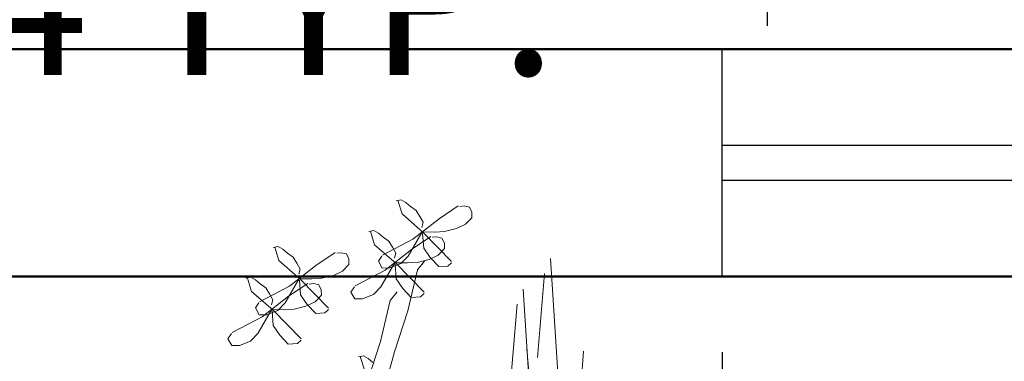
# Model space of a CAD drawing. Units: inches. Extents: x 89 to 490, y -59 to 378.
# Tile 6 of 20: x 300 to 339, y 1 to 15. Entities that reach past the tile are written whole.
import ezdxf

# ---------------------------------------------------------------- set-up
doc = ezdxf.new("R2010")
doc.units = ezdxf.units.IN
doc.header["$MEASUREMENT"] = 0
for name, color, linetype, lineweight in [('A-ANNO-DIMS', 2, 'Continuous', 18), ('L-PLNT', 94, 'Continuous', 18), ('Outer Walls', 12, 'Continuous', 50), ('Windows', 171, 'Continuous', 25)]:
    doc.layers.add(name, color=color, linetype=linetype, lineweight=lineweight)
doc.layers.add('fl', color=73, linetype='Continuous', lineweight=9, true_color=0xa3d166)
doc.styles.get("Standard").update_dxf_attribs({"font": 'arial.ttf'})
doc.dimstyles.get("Standard").update_dxf_attribs({"dimtxt": 6, "dimasz": 4, "dimexe": 3, "dimexo": 3, "dimgap": 0.09, "dimtad": 0, "dimtih": 1, "dimtoh": 1, "dimdec": 1, "dimzin": 0, "dimdsep": 46, "dimlunit": 3, "dimtxsty": 'Standard', "dimcen": 0.09, "dimadec": 0, "dimazin": 0, "dimtfac": 1, "dimtdec": 1, "dimtofl": 0, "dimtmove": 0, "dimatfit": 3, "dimfxl": 1, "dimtolj": 1, "dimtzin": 0, "dimarcsym": 0})

# ---------------------------------------------------------------- blocks, each defined once
blk = doc.blocks.new('Window')
for p, q in [((516.369, 95.253), (588.369, 95.253)), ((588.369, 93.853), (516.369, 93.853))]:
    blk.add_line(p, q)
blk.add_lwpolyline([(588.369, 99.053), (588.369, 90.053), (516.369, 90.053), (516.369, 99.053)], close=True)
blk = doc.blocks.new('Plantation')
at = {"layer": 'fl'}
for p, q in [((538.643, 42.607), (538.842, 42.647)), ((538.71, 42.613), (538.874, 42.084)), ((538.842, 42.647), (539.026, 42.541)), ((539.026, 42.541), (539.211, 42.38)), ((538.874, 42.084), (539.726, 41.335)), ((539.211, 42.38), (539.432, 42.22)), ((539.432, 42.22), (539.581, 41.986)), ((540.339, 41.891), (541.099, 42.403)), ((541.339, 42.399), (541.157, 42.378)), ((541.54, 42.348), (541.339, 42.399)), ((541.634, 42.149), (541.54, 42.348)), ((541.638, 41.931), (541.634, 42.149)), ((539.297, 41.078), (540.339, 41.891)), ((539.581, 41.986), (539.713, 41.752)), ((539.713, 41.752), (539.662, 41.55)), ((541.388, 41.672), (541.638, 41.931)), ((537.559, 41.389), (537.758, 41.429)), ((537.626, 41.395), (537.79, 40.866)), ((537.758, 41.429), (537.942, 41.323)), ((537.942, 41.323), (538.127, 41.162)), ((539.118, 40.412), (539.665, 41.35)), ((539.684, 41.314), (539.731, 40.732)), ((539.72, 41.369), (540.175, 41.359)), ((539.726, 41.335), (540.834, 40.206)), ((540.175, 41.359), (540.556, 41.384)), ((540.556, 41.384), (541.027, 41.501)), ((541.027, 41.501), (541.388, 41.672)), ((538.103, 40.454), (539.297, 41.078)), ((538.127, 41.162), (538.348, 41.002)), ((538.348, 41.002), (538.498, 40.768)), ((539.255, 40.673), (540.015, 41.185)), ((540.255, 41.181), (540.073, 41.16)), ((540.456, 41.13), (540.255, 41.181)), ((540.55, 40.931), (540.456, 41.13)), ((540.554, 40.713), (540.55, 40.931)), ((533.775, 40.757), (533.974, 40.796)), ((533.842, 40.763), (534.006, 40.234)), ((533.974, 40.796), (534.158, 40.69)), ((534.158, 40.69), (534.343, 40.53)), ((534.343, 40.53), (534.564, 40.37)), ((535.471, 40.041), (536.231, 40.553)), ((536.471, 40.549), (536.289, 40.527)), ((536.672, 40.498), (536.471, 40.549)), ((537.79, 40.866), (538.642, 40.117)), ((538.213, 39.86), (539.255, 40.673)), ((538.498, 40.768), (538.629, 40.534)), ((538.629, 40.534), (538.578, 40.332)), ((539.731, 40.732), (539.992, 40.354)), ((540.304, 40.454), (540.554, 40.713)), ((534.006, 40.234), (534.858, 39.485)), ((534.564, 40.37), (534.713, 40.136)), ((534.713, 40.136), (534.845, 39.901)), ((536.766, 40.299), (536.672, 40.498)), ((536.77, 40.08), (536.766, 40.299)), ((538.081, 40.412), (537.939, 40.209)), ((537.939, 40.209), (538.089, 39.939)), ((538.034, 39.194), (538.581, 40.132)), ((538.636, 40.151), (539.091, 40.141)), ((538.832, 40.116), (539.118, 40.412)), ((539.091, 40.141), (539.472, 40.166)), ((539.472, 40.166), (539.943, 40.283)), ((539.484, 39.869), (539.764, 40.219)), ((539.943, 40.283), (540.304, 40.454)), ((539.992, 40.354), (540.326, 39.996)), ((540.689, 40.021), (540.832, 40.151)), ((544.751, 40.317), (545.243, 32.557)), ((534.429, 39.227), (535.471, 40.041)), ((534.845, 39.901), (534.794, 39.7)), ((536.159, 39.651), (536.52, 39.821)), ((536.52, 39.821), (536.77, 40.08)), ((537.019, 39.236), (538.213, 39.86)), ((538.089, 39.939), (538.398, 39.944)), ((538.398, 39.944), (538.832, 40.116)), ((538.6, 40.096), (538.647, 39.514)), ((538.642, 40.117), (539.75, 38.988)), ((539.102, 38.251), (539.484, 39.869)), ((540.326, 39.996), (540.689, 40.021)), ((532.691, 39.539), (532.89, 39.578)), ((532.758, 39.545), (532.922, 39.016)), ((532.89, 39.578), (533.074, 39.472)), ((533.074, 39.472), (533.259, 39.312)), ((534.25, 38.562), (534.797, 39.5)), ((534.816, 39.464), (534.863, 38.882)), ((534.851, 39.519), (535.306, 39.509)), ((534.858, 39.485), (535.966, 38.356)), ((535.306, 39.509), (535.688, 39.534)), ((535.688, 39.534), (536.159, 39.651)), ((538.647, 39.514), (538.908, 39.136)), ((544.235, 36.397), (544.509, 39.729)), ((532.922, 39.016), (533.774, 38.267)), ((533.235, 38.603), (534.429, 39.227)), ((533.259, 39.312), (533.48, 39.152)), ((533.48, 39.152), (533.629, 38.918)), ((534.387, 38.823), (535.147, 39.335)), ((535.387, 39.331), (535.205, 39.309)), ((535.588, 39.28), (535.387, 39.331)), ((535.682, 39.081), (535.588, 39.28)), ((535.686, 38.862), (535.682, 39.081)), ((536.997, 39.194), (536.855, 38.991)), ((536.855, 38.991), (537.005, 38.721)), ((537.748, 38.898), (538.034, 39.194)), ((538.4, 38.651), (538.68, 39.001)), ((538.908, 39.136), (539.242, 38.778)), ((543.667, 39.099), (544.159, 31.339)), ((533.345, 38.009), (534.387, 38.823)), ((533.629, 38.918), (533.761, 38.683)), ((533.761, 38.683), (533.71, 38.482)), ((534.863, 38.882), (535.124, 38.504)), ((535.075, 38.433), (535.436, 38.603)), ((535.436, 38.603), (535.686, 38.862)), ((537.005, 38.721), (537.314, 38.726)), ((537.314, 38.726), (537.748, 38.898)), ((538.018, 37.033), (538.4, 38.651)), ((539.242, 38.778), (539.605, 38.803)), ((539.605, 38.803), (539.748, 38.932)), ((533.213, 38.562), (533.071, 38.359)), ((533.071, 38.359), (533.221, 38.088)), ((533.166, 37.344), (533.713, 38.282)), ((533.53, 38.094), (533.964, 38.265)), ((533.732, 38.246), (533.779, 37.664)), ((533.768, 38.301), (534.223, 38.291)), ((533.774, 38.267), (534.882, 37.138)), ((533.964, 38.265), (534.25, 38.562)), ((534.223, 38.291), (534.604, 38.316)), ((534.604, 38.316), (535.075, 38.433)), ((535.124, 38.504), (535.458, 38.146)), ((535.821, 38.17), (535.964, 38.3)), ((538.574, 36.629), (539.102, 38.251)), ((543.151, 35.179), (543.425, 38.511)), ((532.151, 37.385), (533.345, 38.009)), ((533.221, 38.088), (533.53, 38.094)), ((535.458, 38.146), (535.821, 38.17)), ((533.779, 37.664), (534.04, 37.286)), ((532.129, 37.344), (531.987, 37.141)), ((531.987, 37.141), (532.137, 36.87)), ((532.446, 36.876), (532.88, 37.047)), ((532.88, 37.047), (533.166, 37.344)), ((534.04, 37.286), (534.374, 36.928)), ((534.737, 36.952), (534.88, 37.082)), ((537.49, 35.411), (538.018, 37.033)), ((532.137, 36.87), (532.446, 36.876)), ((534.374, 36.928), (534.737, 36.952)), ((538.054, 34.764), (538.574, 36.629)), ((543.813, 36.723), (544.326, 31.159)), ((546.054, 36.651), (545.751, 32.703)), ((537.156, 36.43), (537.356, 36.47)), ((537.223, 36.436), (537.387, 35.907)), ((537.356, 36.47), (537.539, 36.364)), ((537.539, 36.364), (537.724, 36.203))]:
    blk.add_line(p, q, dxfattribs=at)
blk = doc.blocks.new('*D28')
at = {"layer": 'A-ANNO-DIMS', "color": 0, "lineweight": -2, "transparency": 16777216}
for p, q in [((326.431, 33.398), (324.379, 33.398)), ((327.379, 29.398), (327.379, 23.72)), ((326.431, 19.72), (324.379, 19.72)), ((327.379, 19.72), (327.379, 15.72)), ((327.379, 15.72), (323.379, 15.72))]:
    blk.add_line(p, q, dxfattribs=at)
at = {"layer": 'A-ANNO-DIMS', "color": 0, "transparency": 16777216}
for points in [[(326.712, 29.398), (328.046, 29.398), (327.379, 33.398)], [(326.712, 23.72), (328.046, 23.72), (327.379, 19.72)]]:
    blk.add_solid(points, dxfattribs=at)
at = {"layer": 'Defpoints', "color": 0, "transparency": 16777216}
for p in [(329.431, 33.398), (327.379, 19.72), (329.431, 19.72)]:
    blk.add_point(p, dxfattribs=at)
at = {"layer": 'A-ANNO-DIMS', "color": 0, "transparency": 16777216, "insert": (294.517, 15.72), "char_height": 6, "attachment_point": 5}
blk.add_mtext('\\A1;CHAIR 14 TYP.', dxfattribs=at)
blk = doc.blocks.new('*D29')
at = {"layer": 'A-ANNO-DIMS', "color": 0, "lineweight": -2, "transparency": 16777216}
for p, q in [((333.431, 17.668), (338.483, 17.668)), ((342.483, 17.668), (346.483, 17.668)), ((329.431, 16.72), (329.431, 14.668)), ((342.483, 16.72), (342.483, 14.668))]:
    blk.add_line(p, q, dxfattribs=at)
at = {"layer": 'A-ANNO-DIMS', "color": 0, "transparency": 16777216}
for points in [[(333.431, 18.335), (333.431, 17.001), (329.431, 17.668)], [(338.483, 18.335), (338.483, 17.001), (342.483, 17.668)]]:
    blk.add_solid(points, dxfattribs=at)
at = {"layer": 'Defpoints', "color": 0, "transparency": 16777216}
for p in [(329.431, 19.72), (342.483, 19.72), (342.483, 17.668)]:
    blk.add_point(p, dxfattribs=at)
at = {"layer": 'A-ANNO-DIMS', "color": 0, "transparency": 16777216, "insert": (360.893, 17.668), "char_height": 6, "attachment_point": 5}
blk.add_mtext('\\A1;13 TYP.', dxfattribs=at)
blk = doc.blocks.new('*D36')
at = {"layer": 'A-ANNO-DIMS', "color": 0, "lineweight": -2, "transparency": 16777216}
for p, q in [((327.654, 1.741), (327.654, -9.059)), ((399.654, 1.741), (399.654, -9.059)), ((331.654, -6.059), (339.621, -6.059)), ((395.654, -6.059), (387.687, -6.059))]:
    blk.add_line(p, q, dxfattribs=at)
at = {"layer": 'A-ANNO-DIMS', "color": 0, "transparency": 16777216}
for points in [[(331.654, -5.392), (331.654, -6.725), (327.654, -6.059)], [(395.654, -5.392), (395.654, -6.725), (399.654, -6.059)]]:
    blk.add_solid(points, dxfattribs=at)
at = {"layer": 'Defpoints', "color": 0, "transparency": 16777216}
for p in [(327.654, 4.741), (399.654, 4.741), (399.654, -6.059)]:
    blk.add_point(p, dxfattribs=at)
at = {"layer": 'A-ANNO-DIMS', "color": 0, "transparency": 16777216, "insert": (363.654, -6.059), "char_height": 6, "attachment_point": 5}
blk.add_mtext('\\A1;WINDOW 72', dxfattribs=at)
blk = doc.blocks.new('*D48')
at = {"layer": 'A-ANNO-DIMS', "color": 0, "lineweight": -2, "transparency": 16777216}
for p, q in [((127.441, 10.741), (127.441, -49.809)), ((459.441, -29.659), (459.441, -49.809)), ((131.441, -46.809), (286.756, -46.809)), ((455.441, -46.809), (300.127, -46.809))]:
    blk.add_line(p, q, dxfattribs=at)
at = {"layer": 'A-ANNO-DIMS', "color": 0, "transparency": 16777216}
for points in [[(131.441, -46.143), (131.441, -47.476), (127.441, -46.809)], [(455.441, -46.143), (455.441, -47.476), (459.441, -46.809)]]:
    blk.add_solid(points, dxfattribs=at)
at = {"layer": 'Defpoints', "color": 0, "transparency": 16777216}
for p in [(127.441, 13.741), (459.441, -26.659), (459.441, -46.809)]:
    blk.add_point(p, dxfattribs=at)
at = {"layer": 'A-ANNO-DIMS', "color": 0, "transparency": 16777216, "insert": (293.441, -46.809), "char_height": 6, "attachment_point": 5}
blk.add_mtext('\\A1;332', dxfattribs=at)

msp = doc.modelspace()

# ---------------------------------------------------------------- linework, layer by layer
at = {"layer": 'Outer Walls'}
msp.add_line((270.4414, 13.7413), (450.4414, 13.7413), dxfattribs=at)
msp.add_lwpolyline([(214.6478, 67.7413), (265.4414, 67.7413), (265.4414, 4.7413), (459.4414, 4.7413), (459.4414, 353.7413), (127.4414, 353.7413), (127.4414, 13.7413)], dxfattribs=at)

# ---------------------------------------------------------------- block references
at = {"layer": 'L-PLNT'}
msp.add_blockref('Plantation', (-223.8856, -34.8668), dxfattribs=at)
at = {"layer": 'Windows'}
msp.add_blockref('Window', (-188.7147, -85.3119), dxfattribs=at)

# ---------------------------------------------------------------- dimensions: what is measured, and where the dimension line sits
at = {"layer": 'A-ANNO-DIMS'}
dim = msp.add_linear_dim(base=(327.3791, 19.7198), p1=(329.4308, 33.3978), p2=(329.4308, 19.7198), angle=270, text='CHAIR <> TYP.', dimstyle='Standard', override={"dimdec": 0, "dimlfac": 1, "dimrnd": 0, "dimzin": 0, "dimdsep": 46, "dimlunit": 2}, dxfattribs=at)
dim.commit()
dim.dimension.update_dxf_attribs({"geometry": '*D28', "text_midpoint": (294.517, 15.7198)})
for base, p1, p2, text, picture, middle in [((342.4828, 17.668), (329.4308, 19.7198), (342.4828, 19.7198), '<> TYP.', '*D29', (360.8934, 17.668)), ((399.6539, -6.0587), (327.6539, 4.7413), (399.6539, 4.7413), 'WINDOW <>', '*D36', (363.6539, -6.0587))]:
    dim = msp.add_linear_dim(base=base, p1=p1, p2=p2, text=text, dimstyle='Standard', override={"dimdec": 0, "dimlfac": 1, "dimrnd": 0, "dimzin": 0, "dimdsep": 46, "dimlunit": 2}, dxfattribs=at)
    dim.commit()
    dim.dimension.update_dxf_attribs({"geometry": picture, "text_midpoint": middle})
dim = msp.add_linear_dim(base=(459.4414, -46.8094), p1=(127.4414, 13.7413), p2=(459.4414, -26.6594), dimstyle='Standard', override={"dimdec": 0, "dimlfac": 1, "dimrnd": 0, "dimzin": 0, "dimdsep": 46, "dimlunit": 2}, dxfattribs=at)
dim.commit()
dim.dimension.update_dxf_attribs({"geometry": '*D48', "text_midpoint": (293.4414, -46.8094)})

doc.saveas('drawing.dxf')
